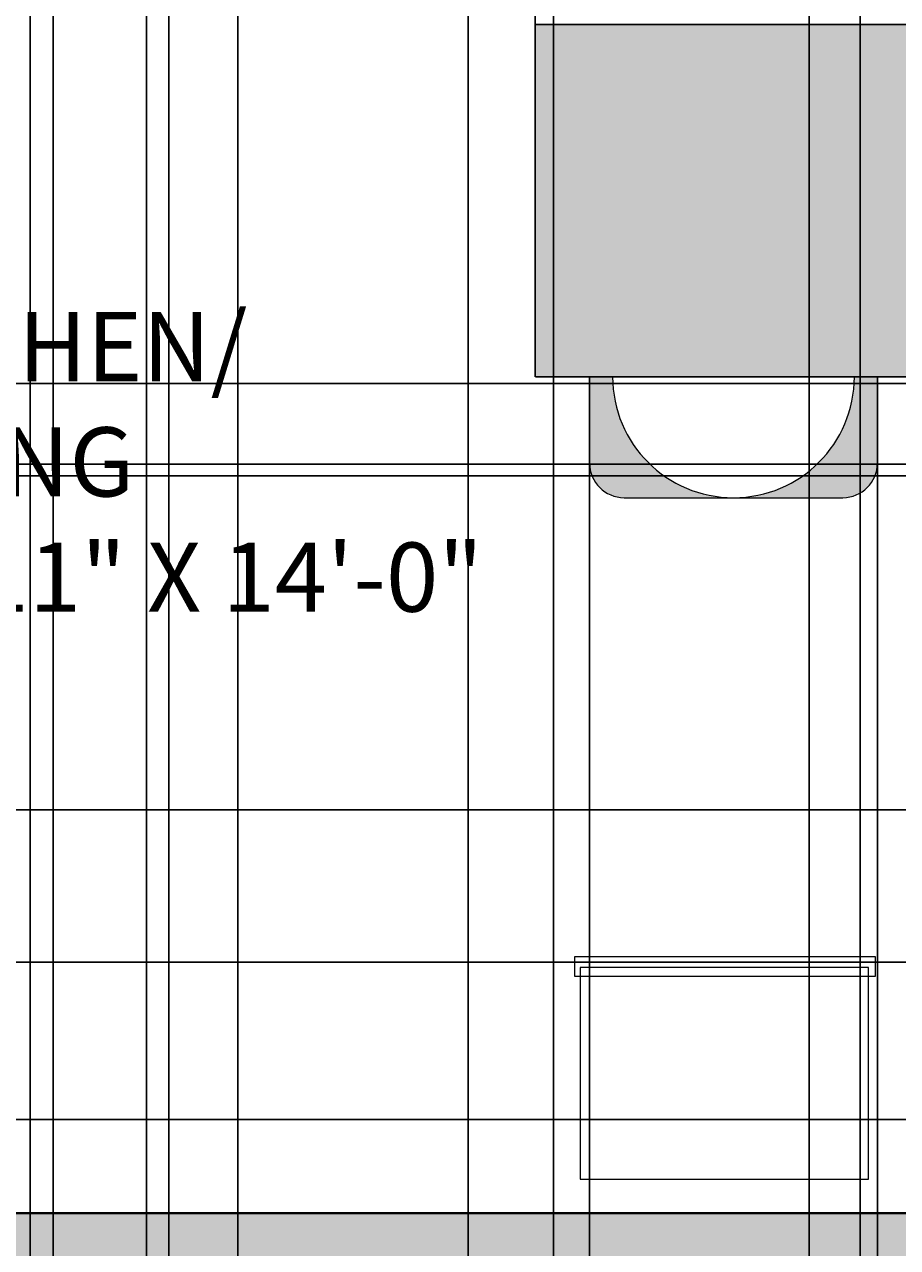
# Model space of a CAD drawing. Units: inches. Extents: x 818 to 1898, y 976 to 2364.
# Tile 82 of 96: x 1439 to 1515, y 1873 to 1979. Entities that reach past the tile are written whole.
import ezdxf

# ---------------------------------------------------------------- set-up
doc = ezdxf.new("R2010")
doc.units = ezdxf.units.IN
doc.header["$LTSCALE"] = 5
doc.header["$MEASUREMENT"] = 0
for name, color, linetype, lineweight in [('A-ANNO-DIMS', 2, 'Continuous', 18), ('A-AREA-IDEN', 7, 'Continuous', 18), ('A-FLOR-CASE', 8, 'Continuous', 18), ('A-FURN', 8, 'Continuous', 18), ('A-FURN-PATT', 8, 'Continuous', 9), ('A-WALL', 7, 'Continuous', 40)]:
    doc.layers.add(name, color=color, linetype=linetype, lineweight=lineweight)
doc.layers.add('A-WALL-PATT', color=251, linetype='Continuous', lineweight=13, true_color=0x636466)
doc.styles.get("Standard").update_dxf_attribs({"font": 'arial.ttf'})
doc.dimstyles.get("Standard").update_dxf_attribs({"dimtxt": 0.18, "dimasz": 0.18, "dimexe": 0.18, "dimexo": 0.0625, "dimgap": 0.09, "dimtad": 0, "dimtih": 1, "dimtoh": 1, "dimdec": 4, "dimzin": 0, "dimdsep": 46, "dimtxsty": 'Standard', "dimcen": 0.09, "dimadec": 0, "dimazin": 0, "dimtfac": 1, "dimtdec": 4, "dimtofl": 0, "dimtmove": 0, "dimatfit": 3, "dimfxl": 1, "dimtolj": 1, "dimtzin": 0, "dimarcsym": 0})

# ---------------------------------------------------------------- blocks, each defined once
blk = doc.blocks.new('*D74')
at = {"layer": 'A-ANNO-DIMS', "color": 0, "lineweight": -2, "ltscale": 5, "transparency": 16777216}
for p, q in [((1590.66, 1940.08), (818.03, 1940.08)), ((818.21, 1939.9), (818.21, 1925.76)), ((818.21, 1911.26), (818.21, 1925.4)), ((1590.66, 1911.08), (818.03, 1911.08))]:
    blk.add_line(p, q, dxfattribs=at)
at = {"layer": 'A-ANNO-DIMS', "color": 0, "ltscale": 5, "transparency": 16777216}
for points in [[(818.18, 1939.9), (818.24, 1939.9), (818.21, 1940.08)], [(818.18, 1911.26), (818.24, 1911.26), (818.21, 1911.08)]]:
    blk.add_solid(points, dxfattribs=at)
at = {"layer": 'Defpoints', "color": 0, "ltscale": 5, "transparency": 16777216}
for p in [(818.21, 1940.08), (1590.73, 1940.08), (1590.73, 1911.08)]:
    blk.add_point(p, dxfattribs=at)
at = {"layer": 'A-ANNO-DIMS', "color": 0, "ltscale": 5, "transparency": 16777216, "insert": (818.21, 1925.58), "char_height": 0.18, "attachment_point": 5}
blk.add_mtext('\\A1;29', dxfattribs=at)
blk = doc.blocks.new('*D85')
at = {"layer": 'A-ANNO-DIMS', "color": 0, "lineweight": -2, "ltscale": 5, "transparency": 16777216}
for p, q in [((1258.79, 2053.08), (1897.92, 2053.08)), ((1897.74, 2052.9), (1897.74, 1876.76)), ((1897.74, 1700.26), (1897.74, 1876.4)), ((1258.79, 1700.08), (1897.92, 1700.08))]:
    blk.add_line(p, q, dxfattribs=at)
at = {"layer": 'A-ANNO-DIMS', "color": 0, "ltscale": 5, "transparency": 16777216}
for points in [[(1897.71, 2052.9), (1897.77, 2052.9), (1897.74, 2053.08)], [(1897.71, 1700.26), (1897.77, 1700.26), (1897.74, 1700.08)]]:
    blk.add_solid(points, dxfattribs=at)
at = {"layer": 'Defpoints', "color": 0, "ltscale": 5, "transparency": 16777216}
for p in [(1258.73, 2053.08), (1897.74, 2053.08), (1258.73, 1700.08)]:
    blk.add_point(p, dxfattribs=at)
at = {"layer": 'A-ANNO-DIMS', "color": 0, "ltscale": 5, "transparency": 16777216, "insert": (1897.74, 1876.58), "char_height": 0.18, "attachment_point": 5}
blk.add_mtext('\\A1;353', dxfattribs=at)
blk = doc.blocks.new('*D99')
at = {"layer": 'A-ANNO-DIMS', "color": 0, "lineweight": -2, "ltscale": 5, "transparency": 16777216}
for p, q in [((1391.88, 1071.12), (1391.88, 2363.87)), ((1392.06, 2363.69), (1420.45, 2363.69)), ((1449.64, 2363.69), (1421.24, 2363.69)), ((1449.82, 1071.12), (1449.82, 2363.87))]:
    blk.add_line(p, q, dxfattribs=at)
at = {"layer": 'A-ANNO-DIMS', "color": 0, "ltscale": 5, "transparency": 16777216}
for points in [[(1392.06, 2363.72), (1392.06, 2363.66), (1391.88, 2363.69)], [(1449.64, 2363.72), (1449.64, 2363.66), (1449.82, 2363.69)]]:
    blk.add_solid(points, dxfattribs=at)
at = {"layer": 'Defpoints', "color": 0, "ltscale": 5, "transparency": 16777216}
for p in [(1449.82, 2363.69), (1391.88, 1071.06), (1449.82, 1071.06)]:
    blk.add_point(p, dxfattribs=at)
at = {"layer": 'A-ANNO-DIMS', "color": 0, "ltscale": 5, "transparency": 16777216, "insert": (1420.85, 2363.69), "char_height": 0.18, "attachment_point": 5}
blk.add_mtext('\\A1;57.94', dxfattribs=at)
blk = doc.blocks.new('*D100')
at = {"layer": 'A-ANNO-DIMS', "color": 0, "lineweight": -2, "ltscale": 5, "transparency": 16777216}
for p, q in [((1449.82, 1071.12), (1449.82, 2363.87)), ((1450, 2363.69), (1478.17, 2363.69)), ((1507.12, 2363.69), (1478.95, 2363.69)), ((1507.3, 1071.12), (1507.3, 2363.87))]:
    blk.add_line(p, q, dxfattribs=at)
at = {"layer": 'A-ANNO-DIMS', "color": 0, "ltscale": 5, "transparency": 16777216}
for points in [[(1450, 2363.72), (1450, 2363.66), (1449.82, 2363.69)], [(1507.12, 2363.72), (1507.12, 2363.66), (1507.3, 2363.69)]]:
    blk.add_solid(points, dxfattribs=at)
at = {"layer": 'Defpoints', "color": 0, "ltscale": 5, "transparency": 16777216}
for p in [(1507.3, 2363.69), (1449.82, 1071.06), (1507.3, 1071.06)]:
    blk.add_point(p, dxfattribs=at)
at = {"layer": 'A-ANNO-DIMS', "color": 0, "ltscale": 5, "transparency": 16777216, "insert": (1478.56, 2363.69), "char_height": 0.18, "attachment_point": 5}
blk.add_mtext('\\A1;57.48', dxfattribs=at)
blk = doc.blocks.new('*D101')
at = {"layer": 'A-ANNO-DIMS', "color": 0, "lineweight": -2, "ltscale": 5, "transparency": 16777216}
for p, q in [((1507.3, 1071.12), (1507.3, 2363.87)), ((1507.48, 2363.69), (1536, 2363.69)), ((1565.3, 2363.69), (1536.78, 2363.69)), ((1565.48, 1071.12), (1565.48, 2363.87))]:
    blk.add_line(p, q, dxfattribs=at)
at = {"layer": 'A-ANNO-DIMS', "color": 0, "ltscale": 5, "transparency": 16777216}
for points in [[(1507.48, 2363.72), (1507.48, 2363.66), (1507.3, 2363.69)], [(1565.3, 2363.72), (1565.3, 2363.66), (1565.48, 2363.69)]]:
    blk.add_solid(points, dxfattribs=at)
at = {"layer": 'Defpoints', "color": 0, "ltscale": 5, "transparency": 16777216}
for p in [(1565.48, 2363.69), (1507.3, 1071.06), (1565.48, 1071.06)]:
    blk.add_point(p, dxfattribs=at)
at = {"layer": 'A-ANNO-DIMS', "color": 0, "ltscale": 5, "transparency": 16777216, "insert": (1536.39, 2363.69), "char_height": 0.18, "attachment_point": 5}
blk.add_mtext('\\A1;58.19', dxfattribs=at)
blk = doc.blocks.new('*D121')
at = {"layer": 'A-ANNO-DIMS', "color": 0, "lineweight": -2, "ltscale": 5, "transparency": 16777216}
for p, q in [((1766.29, 1884.2), (818.03, 1884.2)), ((818.21, 1884.02), (818.21, 1841.14)), ((818.21, 1797.9), (818.21, 1840.78)), ((1766.29, 1797.72), (818.03, 1797.72))]:
    blk.add_line(p, q, dxfattribs=at)
at = {"layer": 'A-ANNO-DIMS', "color": 0, "ltscale": 5, "transparency": 16777216}
for points in [[(818.18, 1884.02), (818.24, 1884.02), (818.21, 1884.2)], [(818.18, 1797.9), (818.24, 1797.9), (818.21, 1797.72)]]:
    blk.add_solid(points, dxfattribs=at)
at = {"layer": 'Defpoints', "color": 0, "ltscale": 5, "transparency": 16777216}
for p in [(818.21, 1884.2), (1766.35, 1884.2), (1766.35, 1797.72)]:
    blk.add_point(p, dxfattribs=at)
at = {"layer": 'A-ANNO-DIMS', "color": 0, "ltscale": 5, "transparency": 16777216, "insert": (818.21, 1840.96), "char_height": 0.18, "attachment_point": 5}
blk.add_mtext('\\A1;86.49', dxfattribs=at)
blk = doc.blocks.new('*D161')
at = {"layer": 'A-ANNO-DIMS', "color": 0, "lineweight": -2, "ltscale": 5, "transparency": 16777216}
for p, q in [((1429.23, 1876.14), (1429.23, 2363.87)), ((1429.41, 2363.69), (1509.59, 2363.69)), ((1590.55, 2363.69), (1510.36, 2363.69)), ((1590.73, 1876.14), (1590.73, 2363.87))]:
    blk.add_line(p, q, dxfattribs=at)
at = {"layer": 'A-ANNO-DIMS', "color": 0, "ltscale": 5, "transparency": 16777216}
for points in [[(1429.41, 2363.72), (1429.41, 2363.66), (1429.23, 2363.69)], [(1590.55, 2363.72), (1590.55, 2363.66), (1590.73, 2363.69)]]:
    blk.add_solid(points, dxfattribs=at)
at = {"layer": 'Defpoints', "color": 0, "ltscale": 5, "transparency": 16777216}
for p in [(1590.73, 2363.69), (1429.23, 1876.08), (1590.73, 1876.08)]:
    blk.add_point(p, dxfattribs=at)
at = {"layer": 'A-ANNO-DIMS', "color": 0, "ltscale": 5, "transparency": 16777216, "insert": (1509.98, 2363.69), "char_height": 0.18, "attachment_point": 5}
blk.add_mtext('\\A1;161.5', dxfattribs=at)
blk = doc.blocks.new('*D169')
at = {"layer": 'A-ANNO-DIMS', "color": 0, "lineweight": -2, "ltscale": 5, "transparency": 16777216}
for p, q in [((1441.73, 1600.14), (1441.73, 2363.87)), ((1441.91, 2363.69), (1459.51, 2363.69)), ((1477.55, 2363.69), (1459.94, 2363.69)), ((1477.73, 1600.14), (1477.73, 2363.87))]:
    blk.add_line(p, q, dxfattribs=at)
at = {"layer": 'A-ANNO-DIMS', "color": 0, "ltscale": 5, "transparency": 16777216}
for points in [[(1441.91, 2363.72), (1441.91, 2363.66), (1441.73, 2363.69)], [(1477.55, 2363.72), (1477.55, 2363.66), (1477.73, 2363.69)]]:
    blk.add_solid(points, dxfattribs=at)
at = {"layer": 'Defpoints', "color": 0, "ltscale": 5, "transparency": 16777216}
for p in [(1477.73, 2363.69), (1441.73, 1600.08), (1477.73, 1600.08)]:
    blk.add_point(p, dxfattribs=at)
at = {"layer": 'A-ANNO-DIMS', "color": 0, "ltscale": 5, "transparency": 16777216, "insert": (1459.73, 2363.69), "char_height": 0.18, "attachment_point": 5}
blk.add_mtext('\\A1;36', dxfattribs=at)
blk = doc.blocks.new('*D196')
at = {"layer": 'A-ANNO-DIMS', "color": 0, "lineweight": -2, "ltscale": 5, "transparency": 16777216}
for p, q in [((1439.73, 1526.73), (1439.73, 2363.87)), ((1439.91, 2363.69), (1448.51, 2363.69)), ((1457.55, 2363.69), (1448.94, 2363.69)), ((1457.73, 1526.73), (1457.73, 2363.87))]:
    blk.add_line(p, q, dxfattribs=at)
at = {"layer": 'A-ANNO-DIMS', "color": 0, "ltscale": 5, "transparency": 16777216}
for points in [[(1439.91, 2363.72), (1439.91, 2363.66), (1439.73, 2363.69)], [(1457.55, 2363.72), (1457.55, 2363.66), (1457.73, 2363.69)]]:
    blk.add_solid(points, dxfattribs=at)
at = {"layer": 'Defpoints', "color": 0, "ltscale": 5, "transparency": 16777216}
for p in [(1457.73, 2363.69), (1439.73, 1526.67), (1457.73, 1526.67)]:
    blk.add_point(p, dxfattribs=at)
at = {"layer": 'A-ANNO-DIMS', "color": 0, "ltscale": 5, "transparency": 16777216, "insert": (1448.73, 2363.69), "char_height": 0.18, "attachment_point": 5}
blk.add_mtext('\\A1;18', dxfattribs=at)
blk = doc.blocks.new('*D206')
at = {"layer": 'A-ANNO-DIMS', "color": 0, "lineweight": -2, "ltscale": 5, "transparency": 16777216}
for p, q in [((1590.66, 1911.08), (818.03, 1911.08)), ((818.21, 1910.9), (818.21, 1893.76)), ((818.21, 1876.26), (818.21, 1893.4)), ((1590.66, 1876.08), (818.03, 1876.08))]:
    blk.add_line(p, q, dxfattribs=at)
at = {"layer": 'A-ANNO-DIMS', "color": 0, "ltscale": 5, "transparency": 16777216}
for points in [[(818.18, 1910.9), (818.24, 1910.9), (818.21, 1911.08)], [(818.18, 1876.26), (818.24, 1876.26), (818.21, 1876.08)]]:
    blk.add_solid(points, dxfattribs=at)
at = {"layer": 'Defpoints', "color": 0, "ltscale": 5, "transparency": 16777216}
for p in [(818.21, 1911.08), (1590.73, 1911.08), (1590.73, 1876.08)]:
    blk.add_point(p, dxfattribs=at)
at = {"layer": 'A-ANNO-DIMS', "color": 0, "ltscale": 5, "transparency": 16777216, "insert": (818.21, 1893.58), "char_height": 0.18, "attachment_point": 5}
blk.add_mtext('\\A1;35', dxfattribs=at)
blk = doc.blocks.new('*D211')
at = {"layer": 'A-ANNO-DIMS', "color": 0, "lineweight": -2, "ltscale": 5, "transparency": 16777216}
for p, q in [((1599.66265, 1948.078237), (818.025912, 1948.078237)), ((818.205912, 1947.898237), (818.205912, 1944.758237)), ((818.205912, 1941.258237), (818.205912, 1944.398237)), ((1599.66265, 1941.078237), (818.025912, 1941.078237))]:
    blk.add_line(p, q, dxfattribs=at)
at = {"layer": 'A-ANNO-DIMS', "color": 0, "ltscale": 5, "transparency": 16777216}
for points in [[(818.175912, 1947.898237), (818.235912, 1947.898237), (818.205912, 1948.078237)], [(818.175912, 1941.258237), (818.235912, 1941.258237), (818.205912, 1941.078237)]]:
    blk.add_solid(points, dxfattribs=at)
at = {"layer": 'Defpoints', "color": 0, "ltscale": 5, "transparency": 16777216}
for p in [(818.205912, 1948.078237), (1599.72515, 1948.078237), (1599.72515, 1941.078237)]:
    blk.add_point(p, dxfattribs=at)
at = {"layer": 'A-ANNO-DIMS', "color": 0, "ltscale": 5, "transparency": 16777216, "insert": (818.205912, 1944.578237), "char_height": 0.18, "attachment_point": 5}
blk.add_mtext('\\A1;7', dxfattribs=at)
blk = doc.blocks.new('*D215')
at = {"layer": 'A-ANNO-DIMS', "color": 0, "lineweight": -2, "ltscale": 5, "transparency": 16777216}
for p, q in [((1590.66, 1876.08), (818.03, 1876.08)), ((818.21, 1875.9), (818.21, 1781.76)), ((818.21, 1687.26), (818.21, 1781.4)), ((1511.66, 1687.08), (818.03, 1687.08))]:
    blk.add_line(p, q, dxfattribs=at)
at = {"layer": 'A-ANNO-DIMS', "color": 0, "ltscale": 5, "transparency": 16777216}
for points in [[(818.18, 1875.9), (818.24, 1875.9), (818.21, 1876.08)], [(818.18, 1687.26), (818.24, 1687.26), (818.21, 1687.08)]]:
    blk.add_solid(points, dxfattribs=at)
at = {"layer": 'Defpoints', "color": 0, "ltscale": 5, "transparency": 16777216}
for p in [(818.21, 1876.08), (1590.73, 1876.08), (1511.73, 1687.08)]:
    blk.add_point(p, dxfattribs=at)
at = {"layer": 'A-ANNO-DIMS', "color": 0, "ltscale": 5, "transparency": 16777216, "insert": (818.21, 1781.58), "char_height": 0.18, "attachment_point": 5}
blk.add_mtext('\\A1;189', dxfattribs=at)
blk = doc.blocks.new('*D238')
at = {"layer": 'A-ANNO-DIMS', "color": 0, "lineweight": -2, "ltscale": 5, "transparency": 16777216}
for p, q in [((1483.55, 1948.72), (1483.55, 2363.87)), ((1483.73, 2363.69), (1516.38, 2363.69)), ((1549.83, 2363.69), (1517.17, 2363.69)), ((1550.01, 1948.72), (1550.01, 2363.87))]:
    blk.add_line(p, q, dxfattribs=at)
at = {"layer": 'A-ANNO-DIMS', "color": 0, "ltscale": 5, "transparency": 16777216}
for points in [[(1483.73, 2363.72), (1483.73, 2363.66), (1483.55, 2363.69)], [(1549.83, 2363.72), (1549.83, 2363.66), (1550.01, 2363.69)]]:
    blk.add_solid(points, dxfattribs=at)
at = {"layer": 'Defpoints', "color": 0, "ltscale": 5, "transparency": 16777216}
for p in [(1550.01, 2363.69), (1483.55, 1948.66), (1550.01, 1948.66)]:
    blk.add_point(p, dxfattribs=at)
at = {"layer": 'A-ANNO-DIMS', "color": 0, "ltscale": 5, "transparency": 16777216, "insert": (1516.78, 2363.69), "char_height": 0.18, "attachment_point": 5}
blk.add_mtext('\\A1;66.47', dxfattribs=at)
blk = doc.blocks.new('*D239')
at = {"layer": 'A-ANNO-DIMS', "color": 0, "lineweight": -2, "ltscale": 5, "transparency": 16777216}
for p, q in [((1483.61, 1979.24), (1897.92, 1979.24)), ((1897.74, 1979.06), (1897.74, 1964.13)), ((1897.74, 1948.84), (1897.74, 1963.77)), ((1483.61, 1948.66), (1897.92, 1948.66))]:
    blk.add_line(p, q, dxfattribs=at)
at = {"layer": 'A-ANNO-DIMS', "color": 0, "ltscale": 5, "transparency": 16777216}
for points in [[(1897.71, 1979.06), (1897.77, 1979.06), (1897.74, 1979.24)], [(1897.71, 1948.84), (1897.77, 1948.84), (1897.74, 1948.66)]]:
    blk.add_solid(points, dxfattribs=at)
at = {"layer": 'Defpoints', "color": 0, "ltscale": 5, "transparency": 16777216}
for p in [(1483.55, 1979.24), (1897.74, 1979.24), (1483.55, 1948.66)]:
    blk.add_point(p, dxfattribs=at)
at = {"layer": 'A-ANNO-DIMS', "color": 0, "ltscale": 5, "transparency": 16777216, "insert": (1897.74, 1963.95), "char_height": 0.18, "attachment_point": 5}
blk.add_mtext('\\A1;30.584', dxfattribs=at)
blk = doc.blocks.new('*D242')
at = {"layer": 'A-ANNO-DIMS', "color": 0, "lineweight": -2, "ltscale": 5, "transparency": 16777216}
for p, q in [((1488.26, 1948.6), (1488.26, 975.66)), ((1513.23, 1948.6), (1513.23, 975.66)), ((1488.44, 975.84), (1500.35, 975.84)), ((1513.05, 975.84), (1501.14, 975.84))]:
    blk.add_line(p, q, dxfattribs=at)
at = {"layer": 'A-ANNO-DIMS', "color": 0, "ltscale": 5, "transparency": 16777216}
for points in [[(1488.44, 975.87), (1488.44, 975.81), (1488.26, 975.84)], [(1513.05, 975.87), (1513.05, 975.81), (1513.23, 975.84)]]:
    blk.add_solid(points, dxfattribs=at)
at = {"layer": 'Defpoints', "color": 0, "ltscale": 5, "transparency": 16777216}
for p in [(1488.26, 1948.66), (1513.23, 1948.66), (1513.23, 975.84)]:
    blk.add_point(p, dxfattribs=at)
at = {"layer": 'A-ANNO-DIMS', "color": 0, "ltscale": 5, "transparency": 16777216, "insert": (1500.74, 975.84), "char_height": 0.18, "attachment_point": 5}
blk.add_mtext('\\A1;24.97', dxfattribs=at)
blk = doc.blocks.new('*D243')
at = {"layer": 'A-ANNO-DIMS', "color": 0, "lineweight": -2, "ltscale": 5, "transparency": 16777216}
for p, q in [((1451.77, 2020.02), (1451.77, 975.66)), ((1590.73, 2020.02), (1590.73, 975.66)), ((1451.95, 975.84), (1520.79, 975.84)), ((1590.55, 975.84), (1521.7, 975.84))]:
    blk.add_line(p, q, dxfattribs=at)
at = {"layer": 'A-ANNO-DIMS', "color": 0, "ltscale": 5, "transparency": 16777216}
for points in [[(1451.95, 975.87), (1451.95, 975.81), (1451.77, 975.84)], [(1590.55, 975.87), (1590.55, 975.81), (1590.73, 975.84)]]:
    blk.add_solid(points, dxfattribs=at)
at = {"layer": 'Defpoints', "color": 0, "ltscale": 5, "transparency": 16777216}
for p in [(1451.77, 2020.08), (1590.73, 2020.08), (1590.73, 975.84)]:
    blk.add_point(p, dxfattribs=at)
at = {"layer": 'A-ANNO-DIMS', "color": 0, "ltscale": 5, "transparency": 16777216, "insert": (1521.25, 975.84), "char_height": 0.18, "attachment_point": 5}
blk.add_mtext('\\A1;138.96', dxfattribs=at)
blk = doc.blocks.new('*D253')
at = {"layer": 'A-ANNO-DIMS', "color": 0, "lineweight": -2, "ltscale": 5, "transparency": 16777216}
for p, q in [((1485.12, 2053.02), (1485.12, 975.66)), ((1538.52, 2053.02), (1538.52, 975.66)), ((1485.3, 975.84), (1511.42, 975.84)), ((1538.34, 975.84), (1512.21, 975.84))]:
    blk.add_line(p, q, dxfattribs=at)
at = {"layer": 'A-ANNO-DIMS', "color": 0, "ltscale": 5, "transparency": 16777216}
for points in [[(1485.3, 975.87), (1485.3, 975.81), (1485.12, 975.84)], [(1538.34, 975.87), (1538.34, 975.81), (1538.52, 975.84)]]:
    blk.add_solid(points, dxfattribs=at)
at = {"layer": 'Defpoints', "color": 0, "ltscale": 5, "transparency": 16777216}
for p in [(1485.12, 2053.08), (1538.52, 2053.08), (1538.52, 975.84)]:
    blk.add_point(p, dxfattribs=at)
at = {"layer": 'A-ANNO-DIMS', "color": 0, "ltscale": 5, "transparency": 16777216, "insert": (1511.82, 975.84), "char_height": 0.18, "attachment_point": 5}
blk.add_mtext('\\A1;53.39', dxfattribs=at)
blk = doc.blocks.new('*D275')
at = {"layer": 'A-ANNO-DIMS', "color": 0, "lineweight": -2, "ltscale": 5, "transparency": 16777216}
for p, q in [((1377.84, 1897.87), (1897.92, 1897.87)), ((1897.74, 1897.69), (1897.74, 1875.99)), ((1897.74, 1853.93), (1897.74, 1875.63)), ((1377.84, 1853.75), (1897.92, 1853.75))]:
    blk.add_line(p, q, dxfattribs=at)
at = {"layer": 'A-ANNO-DIMS', "color": 0, "ltscale": 5, "transparency": 16777216}
for points in [[(1897.71, 1897.69), (1897.77, 1897.69), (1897.74, 1897.87)], [(1897.71, 1853.93), (1897.77, 1853.93), (1897.74, 1853.75)]]:
    blk.add_solid(points, dxfattribs=at)
at = {"layer": 'Defpoints', "color": 0, "ltscale": 5, "transparency": 16777216}
for p in [(1377.78, 1897.87), (1897.74, 1897.87), (1377.78, 1853.75)]:
    blk.add_point(p, dxfattribs=at)
at = {"layer": 'A-ANNO-DIMS', "color": 0, "ltscale": 5, "transparency": 16777216, "insert": (1897.74, 1875.81), "char_height": 0.18, "attachment_point": 5}
blk.add_mtext('\\A1;44.12', dxfattribs=at)
blk = doc.blocks.new('*D281')
at = {"layer": 'A-ANNO-DIMS', "color": 0, "lineweight": -2, "ltscale": 5, "transparency": 16777216}
for p, q in [((1250.3, 1913.7), (1250.3, 2363.87)), ((1250.48, 2363.69), (1420.12, 2363.69)), ((1590.55, 2363.69), (1420.91, 2363.69)), ((1590.73, 2011.14), (1590.73, 2363.87))]:
    blk.add_line(p, q, dxfattribs=at)
at = {"layer": 'A-ANNO-DIMS', "color": 0, "ltscale": 5, "transparency": 16777216}
for points in [[(1250.48, 2363.72), (1250.48, 2363.66), (1250.3, 2363.69)], [(1590.55, 2363.72), (1590.55, 2363.66), (1590.73, 2363.69)]]:
    blk.add_solid(points, dxfattribs=at)
at = {"layer": 'Defpoints', "color": 0, "ltscale": 5, "transparency": 16777216}
for p in [(1590.73, 2363.69), (1590.73, 2011.08), (1250.3, 1913.64)]:
    blk.add_point(p, dxfattribs=at)
at = {"layer": 'A-ANNO-DIMS', "color": 0, "ltscale": 5, "transparency": 16777216, "insert": (1420.51, 2363.69), "char_height": 0.18, "attachment_point": 5}
blk.add_mtext('\\A1;340.4', dxfattribs=at)
blk = doc.blocks.new('*D282')
at = {"layer": 'A-ANNO-DIMS', "color": 0, "lineweight": -2, "ltscale": 5, "transparency": 16777216}
for p, q in [((1422.08, 2081.19), (1897.92, 2081.19)), ((1897.74, 2081.01), (1897.74, 1884.32)), ((1897.74, 1687.26), (1897.74, 1883.95)), ((1463.79, 1687.08), (1897.92, 1687.08))]:
    blk.add_line(p, q, dxfattribs=at)
at = {"layer": 'A-ANNO-DIMS', "color": 0, "ltscale": 5, "transparency": 16777216}
for points in [[(1897.71, 2081.01), (1897.77, 2081.01), (1897.74, 2081.19)], [(1897.71, 1687.26), (1897.77, 1687.26), (1897.74, 1687.08)]]:
    blk.add_solid(points, dxfattribs=at)
at = {"layer": 'Defpoints', "color": 0, "ltscale": 5, "transparency": 16777216}
for p in [(1422.02, 2081.19), (1897.74, 2081.19), (1463.73, 1687.08)]:
    blk.add_point(p, dxfattribs=at)
at = {"layer": 'A-ANNO-DIMS', "color": 0, "ltscale": 5, "transparency": 16777216, "insert": (1897.74, 1884.13), "char_height": 0.18, "attachment_point": 5}
blk.add_mtext('\\A1;394.1', dxfattribs=at)
blk = doc.blocks.new('*D288')
at = {"layer": 'A-ANNO-DIMS', "color": 0, "lineweight": -2, "ltscale": 5, "transparency": 16777216}
for p, q in [((1422.88, 1742.67), (1422.88, 2363.87)), ((1423.06, 2363.69), (1466.91, 2363.69)), ((1511.55, 2363.69), (1467.69, 2363.69)), ((1511.73, 1716.11), (1511.73, 2363.87))]:
    blk.add_line(p, q, dxfattribs=at)
at = {"layer": 'A-ANNO-DIMS', "color": 0, "ltscale": 5, "transparency": 16777216}
for points in [[(1423.06, 2363.72), (1423.06, 2363.66), (1422.88, 2363.69)], [(1511.55, 2363.72), (1511.55, 2363.66), (1511.73, 2363.69)]]:
    blk.add_solid(points, dxfattribs=at)
at = {"layer": 'Defpoints', "color": 0, "ltscale": 5, "transparency": 16777216}
for p in [(1511.73, 2363.69), (1422.88, 1742.61), (1511.73, 1716.05)]:
    blk.add_point(p, dxfattribs=at)
at = {"layer": 'A-ANNO-DIMS', "color": 0, "ltscale": 5, "transparency": 16777216, "insert": (1467.3, 2363.69), "char_height": 0.18, "attachment_point": 5}
blk.add_mtext('\\A1;88.85', dxfattribs=at)

msp = doc.modelspace()

# ---------------------------------------------------------------- hatches: boundary and pattern name
at = {"layer": 'A-FURN-PATT', "ltscale": 5}
h = msp.add_hatch(color=256, dxfattribs=at)
h.dxf.hatch_style = 1
h.paths.add_polyline_path([(1341.9997, 1981.5338), (1317.9034, 2001.8247), (1314.2595, 2001.8247), (1314.2595, 2004.893), (1310.1046, 2008.3917), (1303.9314, 2008.3917), (1303.9314, 1953.0408), (1308.1629, 1953.0408), (1314.2595, 1958.1746), (1314.2595, 1959.6079), (1315.9616, 1959.6079)])
h.paths.add_polyline_path([(1341.9997, 1981.5338), (1315.9616, 1959.6079), (1336.7936, 1959.6079), (1336.7936, 1953.0408), (1345.3966, 1953.0408), (1345.3966, 1959.6079), (1368.0379, 1959.6079)])
h.paths.add_polyline_path([(1402.518, 2008.3917), (1398.8475, 2008.3917), (1398.8475, 2001.8247), (1376.3134, 2001.8247), (1376.3134, 2008.3917), (1373.8948, 2008.3917), (1367.9307, 2003.3695), (1367.9307, 2001.8247), (1366.0961, 2001.8247), (1341.9997, 1981.5338), (1368.0379, 1959.6079), (1375.8366, 1953.0408), (1376.3134, 1953.0408), (1376.3134, 1959.6079), (1398.8475, 1959.6079), (1398.8475, 1953.0408), (1402.518, 1953.0408)])
h.paths.add_polyline_path([(1366.0961, 2001.8247), (1345.3966, 2001.8247), (1345.3966, 2008.3917), (1336.7936, 2008.3917), (1336.7936, 2001.8247), (1317.9034, 2001.8247), (1341.9997, 1981.5338)])
h.paths.add_polyline_path([(1336.7936, 1959.6079), (1315.9616, 1959.6079), (1314.2595, 1958.1746), (1314.2595, 1953.0408), (1336.7936, 1953.0408)], flags=17)
h.paths.add_polyline_path([(1367.9307, 1959.6079), (1345.3966, 1959.6079), (1345.3966, 1953.0408), (1367.9307, 1953.0408)], flags=17)
h.paths.add_polyline_path([(1398.8475, 1959.6079), (1376.3134, 1959.6079), (1376.3134, 1953.0408), (1398.8475, 1953.0408)], flags=17)
h.paths.add_polyline_path([(1368.0379, 1959.6079), (1367.9307, 1959.6079), (1367.9307, 1953.0408), (1375.8366, 1953.0408)], flags=17)
h.paths.add_polyline_path([(1314.2595, 1958.1746), (1308.1629, 1953.0408), (1314.2595, 1953.0408)], flags=17)
h.paths.add_polyline_path([(1315.9616, 1959.6079), (1314.2595, 1959.6079), (1314.2595, 1958.1746)], flags=16)
h.paths.add_polyline_path([(1314.2595, 2008.3917), (1310.1046, 2008.3917), (1314.2595, 2004.893)], flags=17)
h.paths.add_polyline_path([(1336.7936, 2008.3917), (1314.2595, 2008.3917), (1314.2595, 2004.893), (1317.9034, 2001.8247), (1336.7936, 2001.8247)], flags=17)
h.paths.add_polyline_path([(1314.2595, 2004.893), (1314.2595, 2001.8247), (1317.9034, 2001.8247)], flags=16)
h.paths.add_polyline_path([(1367.9307, 2008.3917), (1345.3966, 2008.3917), (1345.3966, 2001.8247), (1366.0961, 2001.8247), (1367.9307, 2003.3695)], flags=17)
h.paths.add_polyline_path([(1398.8475, 2008.3917), (1376.3134, 2008.3917), (1376.3134, 2001.8247), (1398.8475, 2001.8247)], flags=17)
h.paths.add_polyline_path([(1373.8948, 2008.3917), (1367.9307, 2008.3917), (1367.9307, 2003.3695)], flags=17)
h.paths.add_polyline_path([(1367.9307, 2003.3695), (1366.0961, 2001.8247), (1367.9307, 2001.8247)], flags=16)
h.paths.add_polyline_path([(1546.1595, 2044.0782), (1451.7698, 2044.0782), (1451.7698, 2020.0782), (1546.1595, 2020.0782)])
h.paths.add_polyline_path([(1492.0729, 2040.001, 0.431429), (1491.8238, 2040.251), (1491.3087, 2040.251, 0.41521699), (1491.0729, 2040.001)], flags=16)
h.paths.add_polyline_path([(1481.8346, 2039.6036), (1511.886, 2039.6036), (1511.886, 2024.9917), (1481.8346, 2024.9917)], flags=16)
h.paths.add_polyline_path([(1491.0729, 2039.4857), (1491.0729, 2039.501), (1492.0729, 2039.501, -0.41174844), (1491.8401, 2039.251), (1491.8229, 2039.251), (1491.8229, 2039.2509, 0.43259178), (1492.0729, 2039.501), (1491.0729, 2039.501, 0.43260402), (1491.3229, 2039.2509), (1491.3229, 2039.251), (1491.325, 2039.251, -0.41658228)], flags=0)
h.paths.add_polyline_path([(1485.3701, 2030.9622), (1485.3701, 2034.3556, -0.41421356), (1488.3701, 2037.3556), (1490.3421, 2037.3556, -0.07791932), (1491.0729, 2038.751), (1495.0729, 2038.751, -0.31486788), (1496.07, 2037.1201, -0.30166092), (1497.9049, 2034.3556), (1497.9049, 2030.9622, -0.41421356), (1494.9049, 2027.9622), (1488.3701, 2027.9622, -0.41421356)], flags=0)
h.paths.add_polyline_path([(1490.3229, 2035.751, 0.26556482), (1491.3229, 2036.751), (1491.3229, 2037.126), (1491.0729, 2037.126, -0.79141832), (1490.5434, 2037.251, -0.79141832), (1491.0729, 2037.376), (1491.3229, 2037.376), (1491.3229, 2037.751), (1492.0729, 2037.751), (1492.0729, 2037.376), (1492.3229, 2037.376, -0.79141832), (1492.8524, 2037.251, -0.79141832), (1492.3229, 2037.126), (1492.1491, 2037.126, -0.08662632), (1492.5376, 2036.0294, 0.10704809), (1493.0729, 2035.751), (1490.3229, 2035.751)], flags=0)
h.paths.add_polyline_path([(1491.9774, 2037.251, -1), (1491.4184, 2037.251, -1)], flags=0)
h.paths.add_polyline_path([(1500.0743, 2028.6045), (1500.0743, 2029.4074), (1510.8414, 2029.4074), (1510.8414, 2028.6045)], flags=0)
h.paths.add_polyline_path([(1500.0743, 2030.5314), (1500.0743, 2031.3342), (1510.8414, 2031.3342), (1510.8414, 2030.5314)], flags=0)
h.paths.add_polyline_path([(1500.0743, 2032.94), (1500.0743, 2033.7428), (1510.8414, 2033.7428), (1510.8414, 2032.94)], flags=0)
h.paths.add_polyline_path([(1500.0743, 2035.7499), (1500.0743, 2036.5528), (1510.8414, 2036.5528), (1510.8414, 2035.7499)], flags=0)
h.paths.add_polyline_path([(1590.7251, 2044.0782), (1576.1595, 2044.0782), (1576.1595, 2020.0782), (1590.7251, 2020.0782)])
h.paths.add_polyline_path([(1668.4429, 2044.0782), (1599.7251, 2044.0782), (1599.7251, 2020.0782), (1668.4429, 2020.0782)])
h.paths.add_polyline_path([(1621.2588, 2040.001, 0.431429), (1621.0097, 2040.251), (1620.4946, 2040.251, 0.41521699), (1620.2588, 2040.001)], flags=16)
h.paths.add_polyline_path([(1611.0205, 2024.9917), (1611.0205, 2039.6036), (1641.0719, 2039.6036), (1641.0719, 2024.9917)], flags=16)
h.paths.add_polyline_path([(1620.2588, 2039.4857), (1620.2588, 2039.501), (1621.2588, 2039.501, -0.41174844), (1621.026, 2039.251), (1621.0088, 2039.251), (1621.0088, 2039.2509, 0.43259178), (1621.2588, 2039.501), (1620.2588, 2039.501, 0.43260402), (1620.5088, 2039.2509), (1620.5088, 2039.251), (1620.5109, 2039.251, -0.41658228)], flags=0)
h.paths.add_polyline_path([(1614.556, 2030.9622), (1614.556, 2034.3556, -0.41421356), (1617.556, 2037.3556), (1619.528, 2037.3556, -0.07791932), (1620.2588, 2038.751), (1624.2588, 2038.751, -0.31486788), (1625.2559, 2037.1201, -0.30166092), (1627.0908, 2034.3556), (1627.0908, 2030.9622, -0.41421356), (1624.0908, 2027.9622), (1617.556, 2027.9622, -0.41421356)], flags=0)
h.paths.add_polyline_path([(1619.5088, 2035.751, 0.26556482), (1620.5088, 2036.751), (1620.5088, 2037.126), (1620.2588, 2037.126, -0.79141832), (1619.7293, 2037.251, -0.79141832), (1620.2588, 2037.376), (1620.5088, 2037.376), (1620.5088, 2037.751), (1621.2588, 2037.751), (1621.2588, 2037.376), (1621.5088, 2037.376, -0.79141832), (1622.0383, 2037.251, -0.79141832), (1621.5088, 2037.126), (1621.335, 2037.126, -0.08662632), (1621.7235, 2036.0294, 0.10704809), (1622.2588, 2035.751), (1619.5088, 2035.751)], flags=0)
h.paths.add_polyline_path([(1620.6043, 2037.251, -1), (1621.1633, 2037.251, -1)], flags=0)
h.paths.add_polyline_path([(1629.2602, 2028.6045), (1629.2602, 2029.4074), (1640.0273, 2029.4074), (1640.0273, 2028.6045)], flags=0)
h.paths.add_polyline_path([(1629.2602, 2030.5314), (1629.2602, 2031.3342), (1640.0273, 2031.3342), (1640.0273, 2030.5314)], flags=0)
h.paths.add_polyline_path([(1629.2602, 2032.94), (1629.2602, 2033.7428), (1640.0273, 2033.7428), (1640.0273, 2032.94)], flags=0)
h.paths.add_polyline_path([(1629.2602, 2035.7499), (1629.2602, 2036.5528), (1640.0273, 2036.5528), (1640.0273, 2035.7499)], flags=0)
h.paths.add_polyline_path([(1705.7252, 2044.0782), (1698.4429, 2044.0782), (1698.4429, 2020.0782), (1705.7252, 2020.0782)])
h.paths.add_polyline_path([(1705.7252, 1972.0782), (1599.7251, 1972.0782), (1599.7251, 1948.0782), (1705.7252, 1948.0782)])
h.paths.add_polyline_path([(1550.0109, 1979.2444), (1483.5451, 1979.2444), (1483.5451, 1948.6602), (1550.0109, 1948.6602)])
h.paths.add_polyline_path([(1490.2586, 1948.6602), (1488.2586, 1948.6602), (1488.2586, 1941.1742, 0.41421356), (1491.2586, 1938.1742), (1500.7446, 1938.1742, -0.41421356)])
h.paths.add_polyline_path([(1513.2306, 1941.1742), (1513.2306, 1948.6602), (1511.2306, 1948.6602, -0.41421356), (1500.7446, 1938.1742), (1510.2306, 1938.1742, 0.41421356)])
h.paths.add_polyline_path([(1518.778, 1948.6602), (1516.778, 1948.6602), (1516.778, 1941.1742, 0.41421356), (1519.778, 1938.1742), (1529.264, 1938.1742, -0.41421356)])
h.paths.add_polyline_path([(1541.75, 1941.1742), (1541.75, 1948.6602), (1539.75, 1948.6602, -0.41421356), (1529.264, 1938.1742), (1538.75, 1938.1742, 0.41421356)])
h.paths.add_polyline_path([(1590.7251, 1900.0782), (1519.6413, 1900.0782), (1519.6413, 1876.0782), (1590.7251, 1876.0782)])
at = {"layer": 'A-WALL-PATT', "ltscale": 5}
h = msp.add_hatch(color=256, dxfattribs=at)
h.dxf.hatch_style = 1
h.paths.add_polyline_path([(1267.7252, 1928.9218), (1258.7251, 1928.9218), (1258.7251, 1913.6401), (1250.3029, 1913.6401), (1250.3029, 1878.3919), (1258.7251, 1878.3919), (1258.7251, 1862.9652), (1267.7252, 1862.9652)])
h.paths.add_polyline_path([(1267.7252, 1814.9652), (1258.7251, 1814.9652), (1258.7251, 1755.3321), (1267.7252, 1755.3321)])
h.paths.add_polyline_path([(1463.7251, 1696.0782), (1267.7252, 1696.0782), (1267.7252, 1707.3321), (1258.7251, 1707.3321), (1258.7251, 1700.0782), (1251.9333, 1700.0782), (1251.9333, 1687.0782), (1463.7251, 1687.0782)])
h.paths.add_polyline_path([(1714.7252, 1717.3178), (1705.7252, 1717.3178), (1705.7252, 1696.0782), (1599.7251, 1696.0782), (1599.7251, 1790.0782), (1705.7252, 1790.0782), (1705.7252, 1785.6125), (1714.7252, 1785.6125), (1714.7252, 1827.2125), (1705.7252, 1827.2125), (1705.7252, 1802.0782), (1599.7251, 1802.0782), (1599.7251, 1867.0782), (1705.7252, 1867.0782), (1705.7252, 1857.2125), (1714.7252, 1857.2125), (1714.7252, 1930.0316), (1741.8409, 1930.0316), (1741.8409, 1935.0316), (1714.7252, 1935.0316), (1714.7252, 1957.0338), (1741.8409, 1957.0338), (1741.8409, 1962.0338), (1714.7252, 1962.0338), (1705.7252, 1962.0338), (1705.7252, 1948.0782), (1599.7251, 1948.0782), (1599.7251, 1981.0782), (1590.7251, 1981.0782), (1590.7251, 1941.0782), (1620.7252, 1941.0782), (1705.7252, 1941.0782), (1705.7252, 1876.0782), (1599.7251, 1876.0782), (1599.7251, 1911.0782), (1590.7251, 1911.0782), (1590.7251, 1876.0782), (1429.2251, 1876.0782), (1429.2251, 1867.0782), (1511.7251, 1867.0782), (1528.593, 1867.0782), (1595.7252, 1867.0782), (1595.7252, 1773.0782), (1520.7252, 1773.0782), (1520.7252, 1837.5823), (1532.593, 1837.5823), (1532.593, 1867.0782), (1528.593, 1867.0782), (1528.593, 1841.5823), (1511.7251, 1841.5823), (1511.7251, 1744.9714), (1520.7252, 1744.9714), (1520.7252, 1761.0782), (1595.7252, 1761.0782), (1595.7252, 1696.0782), (1520.7252, 1696.0782), (1520.7252, 1716.0454), (1511.7251, 1716.0454), (1511.7251, 1696.0782), (1511.7251, 1687.0782), (1714.7252, 1687.0782)])
h.paths.add_polyline_path([(1714.7252, 2053.0782), (1714.7252, 2081.1881), (1709.7252, 2081.1881), (1709.7252, 2053.0782), (1681.6446, 2053.0782), (1681.6446, 2081.1881), (1676.6446, 2081.1881), (1676.6446, 2053.0782), (1538.5155, 2053.0782), (1538.5155, 2044.0782), (1590.7251, 2044.0782), (1590.7251, 2011.0782), (1599.7251, 2011.0782), (1599.7251, 2044.0782), (1705.7252, 2044.0782), (1705.7252, 2014.5114), (1714.7252, 2014.5114)])
h.paths.add_polyline_path([(1485.1216, 2053.0782), (1422.02, 2053.0782), (1422.02, 2081.1881), (1413.02, 2081.1881), (1413.02, 2053.0782), (1399.6356, 2053.0782), (1399.6356, 2081.1881), (1390.6356, 2081.1881), (1390.6356, 2053.0782), (1388.0315, 2053.0782), (1388.0315, 2044.0782), (1416.2743, 2044.0782), (1485.1216, 2044.0782)])
h.paths.add_polyline_path([(1330.305, 2053.0782), (1258.7251, 2053.0782), (1258.7251, 2019.2871), (1267.7252, 2019.2871), (1267.7252, 2044.0782), (1330.305, 2044.0782)])
h.paths.add_polyline_path([(1258.7251, 2053.0782), (1214.6577, 2053.0782), (1214.6577, 2044.0782), (1258.7251, 2044.0782)])
h.paths.add_polyline_path([(1214.6577, 2053.0782), (1180.349, 2053.0782), (1180.349, 2044.0782), (1214.6577, 2044.0782)])
h.paths.add_polyline_path([(1714.7252, 1639.5782), (1741.8409, 1639.5782), (1741.8409, 1643.5782), (1714.7252, 1643.5782), (1714.7252, 1649.9029), (1705.7252, 1649.9029), (1705.7252, 1600.0782), (1477.7251, 1600.0782), (1477.7251, 1591.0782), (1520.7252, 1591.0782), (1616.7252, 1591.0782), (1616.7252, 1416.6857), (1622.7252, 1416.6857), (1622.7252, 1463.0782), (1624.7252, 1463.0782), (1624.7252, 1467.0782), (1622.7252, 1467.0782), (1622.7252, 1591.0782), (1705.7252, 1591.0782), (1705.7252, 1545.0782), (1714.7252, 1545.0782), (1741.8409, 1545.0782), (1741.8409, 1549.0782), (1714.7252, 1549.0782), (1714.7252, 1593.9175), (1737.8409, 1593.9175), (1737.8409, 1597.9175), (1714.7252, 1597.9175)])
h.paths.add_polyline_path([(1674.9024, 2060.7419), (1714.7045, 2060.7419), (1714.7045, 2073.1061), (1674.9024, 2073.1061)], flags=25)
h.paths.add_polyline_path([(1394.5468, 2061.6618), (1422.2344, 2061.6618), (1422.2344, 2074.0261), (1394.5468, 2074.0261)], flags=24)

# ---------------------------------------------------------------- linework, layer by layer
at = {"layer": 'A-FLOR-CASE'}
msp.add_lwpolyline([(1483.5451, 1979.2444), (1550.0109, 1979.2444), (1550.0109, 1948.6602), (1483.5451, 1948.6602)], close=True, dxfattribs=at)
at = {"layer": 'A-FURN'}
for p, q in [((1490.2586, 1948.6602), (1488.2586, 1948.6602)), ((1488.2586, 1948.6602), (1488.2586, 1941.1742)), ((1513.2306, 1941.1742), (1513.2306, 1948.6602)), ((1491.2586, 1938.1742), (1500.7446, 1938.1742)), ((1500.7446, 1938.1742), (1510.2306, 1938.1742))]:
    msp.add_line(p, q, dxfattribs=at)
for points in [[(1486.9687, 1898.3519), (1513.0405, 1898.3519), (1513.0405, 1896.6229), (1486.9687, 1896.6229)], [(1512.4568, 1897.3936), (1487.4398, 1897.3936), (1487.4398, 1879.0341), (1512.4568, 1879.0341)]]:
    msp.add_lwpolyline(points, close=True, dxfattribs=at)
for centre, radius, start, end in [((1500.7446, 1948.6602), 10.486, 180, 0), ((1491.2586, 1941.1742), 3, 180, 270), ((1510.2306, 1941.1742), 3, 270, 0)]:
    msp.add_arc(centre, radius, start, end, dxfattribs=at)
at = {"layer": 'A-WALL'}
msp.add_line((1429.2251, 1876.0782), (1590.7251, 1876.0782), dxfattribs=at)

# ---------------------------------------------------------------- texts
at = {"layer": 'A-AREA-IDEN', "ltscale": 5, "insert": (1420.8692, 1954.2828), "char_height": 6, "attachment_point": 1}
msp.add_mtext_dynamic_manual_height_columns('KITCHEN/\\PDINING\\P26\'-11" X 14\'-0"', width=118.992422, gutter_width=1, heights=[0], dxfattribs=at)

# ---------------------------------------------------------------- dimensions: what is measured, and where the dimension line sits
at = {"layer": 'A-ANNO-DIMS', "ltscale": 5}
for base, p1, p2, override, picture, middle in [((1590.7251, 2363.6929), (1250.3029, 1913.6401), (1590.7251, 2011.0782), {"dimdec": 1, "dimlfac": 1, "dimrnd": 0, "dimzin": 0, "dimdsep": 46, "dimlunit": 2}, '*D281', (1420.514, 2363.6929)), ((1449.8196, 2363.6929), (1391.8757, 1071.0552), (1449.8196, 1071.0552), {"dimdec": 2, "dimlfac": 1, "dimrnd": 0, "dimzin": 0, "dimdsep": 46, "dimlunit": 2}, '*D99', (1420.8477, 2363.6929)), ((1511.7251, 2363.6929), (1422.8756, 1742.6113), (1511.7251, 1716.0454), {"dimdec": 2, "dimlfac": 1, "dimrnd": 0, "dimzin": 0, "dimdsep": 46, "dimlunit": 2}, '*D288', (1467.3004, 2363.6929)), ((1590.7251, 2363.6929), (1429.2251, 1876.0782), (1590.7251, 1876.0782), {"dimdec": 1, "dimlfac": 1, "dimrnd": 0, "dimzin": 0, "dimdsep": 46, "dimlunit": 2}, '*D161', (1509.9751, 2363.6929)), ((1457.7251, 2363.6929), (1439.7251, 1526.6712), (1457.7251, 1526.6712), {"dimdec": 0, "dimlfac": 1, "dimrnd": 0, "dimzin": 0, "dimdsep": 46, "dimlunit": 2}, '*D196', (1448.7251, 2363.6929)), ((1477.7251, 2363.6929), (1441.7251, 1600.0782), (1477.7251, 1600.0782), {"dimdec": 0, "dimlfac": 1, "dimrnd": 0, "dimzin": 0, "dimdsep": 46, "dimlunit": 2}, '*D169', (1459.7251, 2363.6929)), ((1507.2982, 2363.6929), (1449.8196, 1071.0552), (1507.2982, 1071.0552), {"dimdec": 2, "dimlfac": 1, "dimrnd": 0, "dimzin": 0, "dimdsep": 46, "dimlunit": 2}, '*D100', (1478.5589, 2363.6929)), ((1550.0109, 2363.6929), (1483.5451, 1948.6602), (1550.0109, 1948.6602), {"dimdec": 2, "dimlfac": 1, "dimrnd": 0, "dimzin": 0, "dimdsep": 46, "dimlunit": 2}, '*D238', (1516.778, 2363.6929)), ((1565.4835, 2363.6929), (1507.2982, 1071.0552), (1565.4835, 1071.0552), {"dimdec": 2, "dimlfac": 1, "dimrnd": 0, "dimzin": 0, "dimdsep": 46, "dimlunit": 2}, '*D101', (1536.3908, 2363.6929)), ((1538.5155, 975.8433), (1485.1216, 2053.0782), (1538.5155, 2053.0782), {"dimdec": 2, "dimlfac": 1, "dimrnd": 0, "dimzin": 0, "dimdsep": 46, "dimlunit": 2}, '*D253', (1511.8185, 975.8433)), ((1590.7251, 975.8433), (1451.7698, 2020.0782), (1590.7251, 2020.0782), {"dimdec": 2, "dimlfac": 1, "dimrnd": 0, "dimzin": 0, "dimdsep": 46, "dimlunit": 2}, '*D243', (1521.2475, 975.8433)), ((1513.2306, 975.8433), (1488.2586, 1948.6602), (1513.2306, 1948.6602), {"dimdec": 2, "dimlfac": 1, "dimrnd": 0, "dimzin": 0, "dimdsep": 46, "dimlunit": 2}, '*D242', (1500.7446, 975.8433))]:
    dim = msp.add_linear_dim(base=base, p1=p1, p2=p2, dimstyle='Standard', override=override, dxfattribs=at)
    dim.commit()
    dim.dimension.update_dxf_attribs({"geometry": picture, "text_midpoint": middle})
for base, p1, p2, override, picture, middle in [((1897.736, 2081.1881), (1463.7251, 1687.0782), (1422.02, 2081.1881), {"dimdec": 1, "dimlfac": 1, "dimrnd": 0, "dimzin": 0, "dimdsep": 46, "dimlunit": 2}, '*D282', (1897.736, 1884.1332)), ((1897.736, 2053.0782), (1258.7251, 1700.0782), (1258.7251, 2053.0782), {"dimdec": 0, "dimlfac": 1, "dimrnd": 0, "dimzin": 0, "dimdsep": 46, "dimlunit": 2}, '*D85', (1897.736, 1876.5782)), ((1897.736, 1979.2444), (1483.5451, 1948.6602), (1483.5451, 1979.2444), {"dimdec": 3, "dimlfac": 1, "dimrnd": 0, "dimzin": 0, "dimdsep": 46, "dimlunit": 2}, '*D239', (1897.736, 1963.9523)), ((818.2059, 1948.0782), (1599.7251, 1941.0782), (1599.7251, 1948.0782), {"dimdec": 0, "dimlfac": 1, "dimrnd": 0, "dimzin": 0, "dimdsep": 46, "dimlunit": 2}, '*D211', (818.2059, 1944.5782)), ((818.2059, 1940.0782), (1590.7251, 1911.0782), (1590.7251, 1940.0782), {"dimdec": 0, "dimlfac": 1, "dimrnd": 0, "dimzin": 0, "dimdsep": 46, "dimlunit": 2}, '*D74', (818.2059, 1925.5782)), ((818.2059, 1911.0782), (1590.7251, 1876.0782), (1590.7251, 1911.0782), {"dimdec": 0, "dimlfac": 1, "dimrnd": 0, "dimzin": 0, "dimdsep": 46, "dimlunit": 2}, '*D206', (818.2059, 1893.5782)), ((1897.736, 1897.8663), (1377.7791, 1853.7496), (1377.7791, 1897.8663), {"dimdec": 2, "dimlfac": 1, "dimrnd": 0, "dimzin": 0, "dimdsep": 46, "dimlunit": 2}, '*D275', (1897.736, 1875.808)), ((818.2059, 1884.2031), (1766.3524, 1797.7165), (1766.3524, 1884.2031), {"dimdec": 2, "dimlfac": 1, "dimrnd": 0, "dimzin": 0, "dimdsep": 46, "dimlunit": 2}, '*D121', (818.2059, 1840.9598)), ((818.2059, 1876.0782), (1511.7251, 1687.0782), (1590.7251, 1876.0782), {"dimdec": 0, "dimlfac": 1, "dimrnd": 0, "dimzin": 0, "dimdsep": 46, "dimlunit": 2}, '*D215', (818.2059, 1781.5782))]:
    dim = msp.add_linear_dim(base=base, p1=p1, p2=p2, angle=90, dimstyle='Standard', override=override, dxfattribs=at)
    dim.commit()
    dim.dimension.update_dxf_attribs({"geometry": picture, "text_midpoint": middle})

doc.saveas('drawing.dxf')
